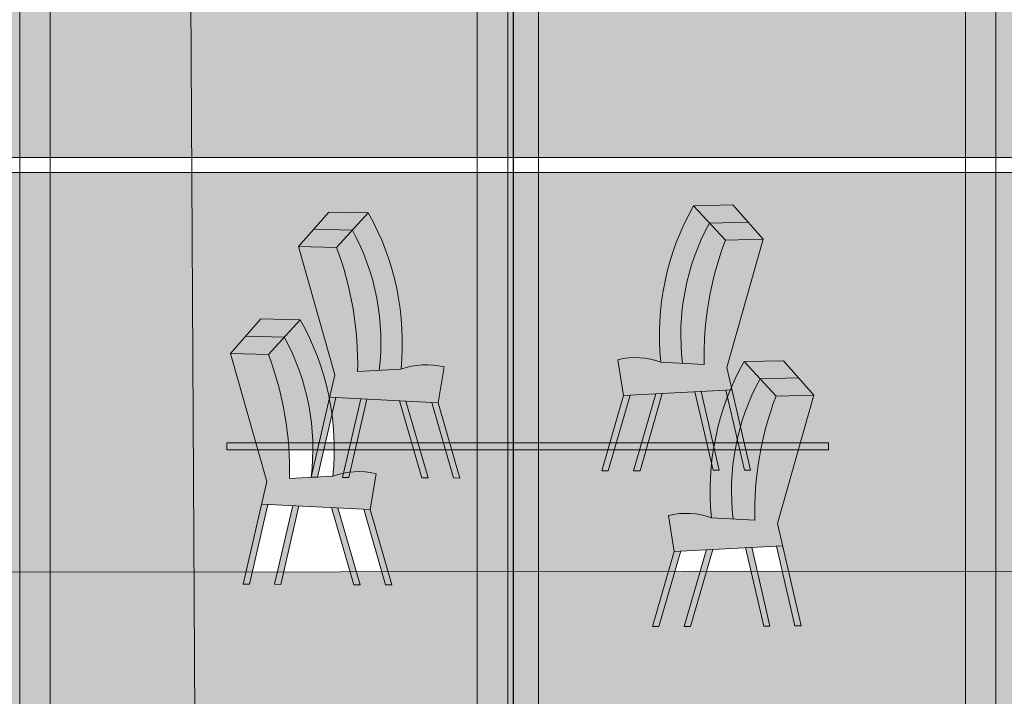
# Model space of a CAD drawing. Units: millimetres. Extents: x 11032 to 26788, y 3406 to 24505.
# Tile 14 of 78: x 17145 to 18758, y 7381 to 8490. Entities that reach past the tile are written whole.
import ezdxf

# ---------------------------------------------------------------- set-up
doc = ezdxf.new("R2010")
doc.units = ezdxf.units.MM
doc.header["$MEASUREMENT"] = 0
for name, color, linetype, lineweight in [('A-ANNO-DIMS', 2, 'Continuous', 18), ('A-FURN', 8, 'Continuous', 13), ('A-FURN-PATT', 8, 'Continuous', 13), ('A-GLAZ', 250, 'Continuous', 20), ('A-WALL-INTR', 8, 'Continuous', 18)]:
    doc.layers.add(name, color=color, linetype=linetype, lineweight=lineweight)
for name, color, linetype, lineweight, true_color in [('A-FNSH-INTR-PATT', 253, 'Continuous', 13, 0xc2b29b), ('A-GLAZ-FRAM-PATT', 250, 'Continuous', 13, 0x262627), ('A-WALL-INTR-PATT', 251, 'Continuous', 13, 0x6c6b6a)]:
    doc.layers.add(name, color=color, linetype=linetype, lineweight=lineweight, true_color=true_color)
doc.styles.get("Standard").update_dxf_attribs({"font": 'arial.ttf'})
doc.dimstyles.get("Standard").update_dxf_attribs({"dimtxt": 150, "dimasz": 100, "dimexe": 10, "dimexo": 5, "dimgap": 5, "dimtad": 0, "dimtih": 1, "dimtoh": 1, "dimdec": 0, "dimzin": 0, "dimdsep": 46, "dimtxsty": 'Standard', "dimcen": 0.09, "dimadec": 0, "dimazin": 0, "dimtfac": 1, "dimtdec": 0, "dimtofl": 0, "dimtmove": 0, "dimatfit": 3, "dimfxl": 1, "dimtolj": 1, "dimtzin": 0, "dimarcsym": 0})

# ---------------------------------------------------------------- blocks, each defined once
blk = doc.blocks.new('DINING-CHAIR-ELEV')
blk.add_line((228.7, 123.4), (51, 132.6))
for points in [[(0, 379.5), (49.4, 435.9), (114.1, 434.5)], [(61.2, 132.1), (30.8, 1.2), (20.5, 1.2), (59.5, 169.3), (0, 379.5), (61.9, 377.9)], [(111.9, 129.5), (82.1, 0.9), (71.8, 1), (101.8, 130)], [(165.3, 126.7), (201.8, 0.3), (212.2, 0.3), (175.8, 126.2)]]:
    blk.add_lwpolyline(points)
for points in [[(218.1, 124), (253.9, 0.1), (264.3, 0), (228.7, 123.4), (238.3, 182.2, 0.148451), (167.5, 178.3), (96.6, 174.5, 0.097012), (61.9, 377.9), (114.1, 434.5, -0.154833), (167.8, 178.5)], [(132, 176.4, 0.156877), (88, 406.2), (24.7, 407.7)]]:
    blk.add_lwpolyline(points, format="xyb")
blk = doc.blocks.new('DINING-TABLE-ELEV')
blk.add_lwpolyline([(0, 0), (986.1, 0), (986.1, 11.1), (0, 11.1)], close=True)
blk = doc.blocks.new('*D36')
at = {"layer": 'A-ANNO-DIMS', "color": 0, "lineweight": -2, "transparency": 16777216}
for p, q in [((12301.3, 17115.9), (12301.3, 24416.9)), ((25397.4, 4466.4), (25397.4, 24416.9)), ((12401.3, 24406.9), (18569.2, 24406.9)), ((25297.4, 24406.9), (19129.5, 24406.9))]:
    blk.add_line(p, q, dxfattribs=at)
at = {"layer": 'A-ANNO-DIMS', "color": 0, "transparency": 16777216}
for points in [[(12401.3, 24423.5), (12401.3, 24390.2), (12301.3, 24406.9)], [(25297.4, 24423.5), (25297.4, 24390.2), (25397.4, 24406.9)]]:
    blk.add_solid(points, dxfattribs=at)
at = {"layer": 'Defpoints', "color": 0, "transparency": 16777216}
for p in [(25397.4, 24406.9), (12301.3, 17110.9), (25397.4, 4461.4)]:
    blk.add_point(p, dxfattribs=at)
at = {"layer": 'A-ANNO-DIMS', "color": 0, "transparency": 16777216, "insert": (18849.3, 24406.9), "char_height": 150, "attachment_point": 5}
blk.add_mtext('\\A1;13096', dxfattribs=at)
blk = doc.blocks.new('*D37')
at = {"layer": 'A-ANNO-DIMS', "color": 0, "lineweight": -2, "transparency": 16777216}
for p, q in [((18087.7, 23450.4), (11334.8, 23450.4)), ((11344.8, 23350.4), (11344.8, 14037.5)), ((11344.8, 4561.4), (11344.8, 13874.3)), ((12927.7, 4461.4), (11334.8, 4461.4))]:
    blk.add_line(p, q, dxfattribs=at)
at = {"layer": 'A-ANNO-DIMS', "color": 0, "transparency": 16777216}
for points in [[(11328.1, 23350.4), (11361.4, 23350.4), (11344.8, 23450.4)], [(11328.1, 4561.4), (11361.4, 4561.4), (11344.8, 4461.4)]]:
    blk.add_solid(points, dxfattribs=at)
at = {"layer": 'Defpoints', "color": 0, "transparency": 16777216}
for p in [(11344.8, 23450.4), (18092.7, 23450.4), (12932.7, 4461.4)]:
    blk.add_point(p, dxfattribs=at)
at = {"layer": 'A-ANNO-DIMS', "color": 0, "transparency": 16777216, "insert": (11344.8, 13955.9), "char_height": 150, "attachment_point": 5}
blk.add_mtext('\\A1;18989', dxfattribs=at)
blk = doc.blocks.new('*D49')
at = {"layer": 'A-ANNO-DIMS', "color": 0, "lineweight": -2, "transparency": 16777216}
for p, q in [((17953.5, 10206.4), (17953.5, 3494.9)), ((14996.4, 6406.4), (14996.4, 3494.9)), ((15096.4, 3504.9), (16244.7, 3504.9)), ((17853.5, 3504.9), (16705.2, 3504.9))]:
    blk.add_line(p, q, dxfattribs=at)
at = {"layer": 'A-ANNO-DIMS', "color": 0, "transparency": 16777216}
for points in [[(15096.4, 3521.6), (15096.4, 3488.2), (14996.4, 3504.9)], [(17853.5, 3521.6), (17853.5, 3488.2), (17953.5, 3504.9)]]:
    blk.add_solid(points, dxfattribs=at)
at = {"layer": 'Defpoints', "color": 0, "transparency": 16777216}
for p in [(17953.5, 10211.4), (14996.4, 6411.4), (17953.5, 3504.9)]:
    blk.add_point(p, dxfattribs=at)
at = {"layer": 'A-ANNO-DIMS', "color": 0, "transparency": 16777216, "insert": (16474.9, 3504.9), "char_height": 150, "attachment_point": 5}
blk.add_mtext('\\A1;2957', dxfattribs=at)
blk = doc.blocks.new('*D50')
at = {"layer": 'A-ANNO-DIMS', "color": 0, "lineweight": -2, "transparency": 16777216}
for p, q in [((19697.4, 16000.7), (19697.4, 3494.9)), ((17953.5, 10206.4), (17953.5, 3494.9)), ((18053.5, 3504.9), (18603.8, 3504.9)), ((19597.4, 3504.9), (19047, 3504.9))]:
    blk.add_line(p, q, dxfattribs=at)
at = {"layer": 'A-ANNO-DIMS', "color": 0, "transparency": 16777216}
for points in [[(18053.5, 3521.6), (18053.5, 3488.2), (17953.5, 3504.9)], [(19597.4, 3521.6), (19597.4, 3488.2), (19697.4, 3504.9)]]:
    blk.add_solid(points, dxfattribs=at)
at = {"layer": 'Defpoints', "color": 0, "transparency": 16777216}
for p in [(19697.4, 16005.7), (17953.5, 10211.4), (19697.4, 3504.9)]:
    blk.add_point(p, dxfattribs=at)
at = {"layer": 'A-ANNO-DIMS', "color": 0, "transparency": 16777216, "insert": (18825.4, 3504.9), "char_height": 150, "attachment_point": 5}
blk.add_mtext('\\A1;1744', dxfattribs=at)
blk = doc.blocks.new('*D57')
at = {"layer": 'A-ANNO-DIMS', "color": 0, "lineweight": -2, "transparency": 16777216}
for p, q in [((14994.7, 7266.4), (14994.7, 24416.9)), ((20894.7, 7266.4), (20894.7, 24416.9)), ((15094.7, 24406.9), (17716, 24406.9)), ((20794.7, 24406.9), (18173.4, 24406.9))]:
    blk.add_line(p, q, dxfattribs=at)
at = {"layer": 'A-ANNO-DIMS', "color": 0, "transparency": 16777216}
for points in [[(15094.7, 24423.5), (15094.7, 24390.2), (14994.7, 24406.9)], [(20794.7, 24423.5), (20794.7, 24390.2), (20894.7, 24406.9)]]:
    blk.add_solid(points, dxfattribs=at)
at = {"layer": 'Defpoints', "color": 0, "transparency": 16777216}
for p in [(20894.7, 24406.9), (14994.7, 7261.4), (20894.7, 7261.4)]:
    blk.add_point(p, dxfattribs=at)
at = {"layer": 'A-ANNO-DIMS', "color": 0, "transparency": 16777216, "insert": (17944.7, 24406.9), "char_height": 150, "attachment_point": 5}
blk.add_mtext('\\A1;5900', dxfattribs=at)
blk = doc.blocks.new('*D66')
at = {"layer": 'A-ANNO-DIMS', "color": 0, "lineweight": -2, "transparency": 16777216}
for p, q in [((16725.9, 10296), (16725.9, 3494.9)), ((19150.9, 10296), (19150.9, 3494.9)), ((16825.9, 3504.9), (17707.6, 3504.9)), ((19050.9, 3504.9), (18169.3, 3504.9))]:
    blk.add_line(p, q, dxfattribs=at)
at = {"layer": 'A-ANNO-DIMS', "color": 0, "transparency": 16777216}
for points in [[(16825.9, 3521.6), (16825.9, 3488.2), (16725.9, 3504.9)], [(19050.9, 3521.6), (19050.9, 3488.2), (19150.9, 3504.9)]]:
    blk.add_solid(points, dxfattribs=at)
at = {"layer": 'Defpoints', "color": 0, "transparency": 16777216}
for p in [(16725.9, 10301), (19150.9, 10301), (19150.9, 3504.9)]:
    blk.add_point(p, dxfattribs=at)
at = {"layer": 'A-ANNO-DIMS', "color": 0, "transparency": 16777216, "insert": (17938.4, 3504.9), "char_height": 150, "attachment_point": 5}
blk.add_mtext('\\A1;2425', dxfattribs=at)
blk = doc.blocks.new('*D69')
at = {"layer": 'A-ANNO-DIMS', "color": 0, "lineweight": -2, "transparency": 16777216}
for p, q in [((13957, 9938), (14057, 9938)), ((14057, 9938), (15432.5, 8991)), ((17944.6, 7261.4), (17944.8, 7261.4)), ((17944.7, 7261.3), (17944.7, 7261.5))]:
    blk.add_line(p, q, dxfattribs=at)
at = {"layer": 'A-ANNO-DIMS', "color": 0, "transparency": 16777216}
blk.add_solid([(15442, 9004.7), (15423.1, 8977.2), (15514.9, 8934.2)], dxfattribs=at)
at = {"layer": 'Defpoints', "color": 0, "transparency": 16777216}
for p in [(15514.9, 8934.2), (17944.7, 7261.4)]:
    blk.add_point(p, dxfattribs=at)
at = {"layer": 'A-ANNO-DIMS', "color": 0, "transparency": 16777216, "insert": (13494, 9938), "char_height": 150, "attachment_point": 5}
blk.add_mtext('\\A1;2X R2950', dxfattribs=at)
blk = doc.blocks.new('*D70')
at = {"layer": 'A-ANNO-DIMS', "color": 0, "lineweight": -2, "transparency": 16777216}
for p, q in [((18044.7, 11901.4), (17944.7, 11901.4)), ((17944.7, 11901.4), (17944.7, 10261.4)), ((17944.6, 7261.4), (17944.8, 7261.4)), ((17944.7, 7261.3), (17944.7, 7261.5))]:
    blk.add_line(p, q, dxfattribs=at)
at = {"layer": 'A-ANNO-DIMS', "color": 0, "transparency": 16777216}
blk.add_solid([(17928, 10261.4), (17961.4, 10261.4), (17944.7, 10161.4)], dxfattribs=at)
at = {"layer": 'Defpoints', "color": 0, "transparency": 16777216}
for p in [(17944.7, 10161.4), (17944.7, 7261.4)]:
    blk.add_point(p, dxfattribs=at)
at = {"layer": 'A-ANNO-DIMS', "color": 0, "transparency": 16777216, "insert": (18345.2, 11901.4), "char_height": 150, "attachment_point": 5}
blk.add_mtext('\\A1;R2900', dxfattribs=at)

msp = doc.modelspace()

# ---------------------------------------------------------------- hatches: boundary and pattern name
at = {"layer": 'A-FNSH-INTR-PATT'}
h = msp.add_hatch(dxfattribs=at)
h.set_pattern_fill('AR-SAND', color=256, scale=30, angle=45, style=0)
h.paths.add_polyline_path([(17894.704, 10061.399), (17417.202, 10027.292), (17426.61, 8264.696), (17894.704, 8264.696)])
h.paths.add_polyline_path([(18694.704, 10011.399), (17994.704, 10061.399), (17994.704, 8264.696), (18694.704, 8264.696)])
h.paths.add_polyline_path([(19494.704, 9712.419, 0.04762013), (19003.004, 9961.399), (18794.704, 9961.399), (18794.704, 8264.696), (19494.704, 8264.696)])
at = {"layer": 'A-FURN-PATT'}
h = msp.add_hatch(color=256, dxfattribs=at)
h.set_gradient(color1=(82, 15, 16), color2=(153, 0, 38), name='CURVED')
h.paths.add_polyline_path([(16952.125, 8119), (16926.017, 8147.32, 0.15687748), (16881.989, 7917.509), (16917.415, 7915.583, -0.09701208)], flags=0)
h.paths.add_polyline_path([(16899.908, 8175.64), (16964.58, 8177.046), (17014.03, 8120.657), (16954.484, 7910.365), (16972.017, 7834.84), (16977.75, 7834.965), (17027.199, 7778.576), (16967.653, 7568.284), (17006.665, 7400.238), (16996.411, 7400.187), (16966.016, 7531.114), (16925.439, 7529.018), (16955.395, 7399.983), (16945.141, 7399.932), (16915.295, 7528.494), (16861.916, 7525.736), (16825.435, 7399.337), (16815.012, 7399.285), (16851.35, 7525.19), (16809.087, 7523.007), (16773.319, 7399.078), (16762.896, 7399.026), (16798.521, 7522.461), (16788.882, 7581.207, -0.14766935), (16859.382, 7577.482, -0.15281323), (16911.41, 7830.579), (16902.125, 7870.575), (16848.746, 7867.817), (16830.506, 7804.617), (16830.506, 7793.515), (16827.302, 7793.515), (16812.265, 7741.418), (16801.842, 7741.366), (16816.893, 7793.515), (16775.261, 7793.515), (16760.15, 7741.159), (16749.727, 7741.107), (16764.853, 7793.515), (16650.704, 7793.515), (16662.994, 7750.932), (16652.571, 7750.983), (16640.296, 7793.515), (16598.663, 7793.515), (16610.879, 7751.191), (16600.455, 7751.242), (16588.255, 7793.515), (16490.425, 7793.515), (16480.749, 7751.837), (16470.495, 7751.888), (16480.159, 7793.515), (16443.833, 7793.515, -0.10940509), (16465.746, 7607.731, -0.14766935), (16536.246, 7611.456), (16526.606, 7552.71), (16562.232, 7429.275), (16551.809, 7429.327), (16516.041, 7553.255), (16473.778, 7555.439), (16510.116, 7429.534), (16499.693, 7429.586), (16463.212, 7555.985), (16409.833, 7558.743), (16379.987, 7430.181), (16369.733, 7430.232), (16394.704, 7537.793), (16394.704, 7559.524), (16359.112, 7561.363), (16328.717, 7430.435), (16318.463, 7430.486), (16344.704, 7543.521), (16344.704, 7643.635), (16302.264, 7793.515), (16205.738, 7793.515), (16227.021, 7719.773), (16216.598, 7719.825), (16195.329, 7793.515), (16153.697, 7793.515), (16174.905, 7720.032), (16164.482, 7720.084), (16143.289, 7793.515), (15844.423, 7793.515), (15844.423, 7804.617), (16140.084, 7804.617), (16128.001, 7846.483), (16191.395, 7843.208), (16201.035, 7901.954, 0.14845082), (16130.184, 7898.102), (16059.333, 7894.25, 0.09701208), (16024.622, 8097.666), (16076.839, 8154.307, -0.15483335), (16130.535, 7898.229, -0.14766935), (16201.035, 7901.954), (16191.395, 7843.208), (16202.533, 7804.617), (16299.12, 7804.617), (16297.929, 7808.825), (16347.378, 7865.214), (16412.05, 7863.808, -0.02954963), (16434.494, 7817.915), (16458.237, 7920.19), (16398.691, 8130.481), (16448.141, 8186.871), (16512.813, 8185.465, -0.15483335), (16566.508, 7929.387, -0.14766935), (16637.008, 7933.112), (16627.369, 7874.366), (16647.499, 7804.617), (16742.939, 7804.617), (16741.107, 8264.696), (17994.704, 8264.696), (17994.704, 7796.661), (18112.02, 7796.661), (18134.447, 7874.366), (18124.807, 7933.112, -0.14766935), (18195.307, 7929.387, -0.15483335), (18249.003, 8185.465), (18313.675, 8186.871), (18363.124, 8130.481), (18303.578, 7920.19), (18311.087, 7887.847, -0.02730168), (18332.016, 7930.161), (18396.688, 7931.567), (18446.137, 7875.177), (18423.905, 7796.661), (18470.25, 7796.661), (18470.25, 7785.559), (18420.761, 7785.559), (18386.591, 7664.886), (18425.604, 7496.839), (18415.35, 7496.788), (18384.955, 7627.716), (18344.377, 7625.62), (18374.333, 7496.584), (18364.079, 7496.533), (18334.233, 7625.095), (18280.854, 7622.338), (18244.373, 7495.938), (18233.95, 7495.887), (18270.288, 7621.792), (18228.026, 7619.608), (18192.257, 7495.679), (18181.834, 7495.628), (18217.46, 7619.062), (18207.82, 7677.808, -0.14766935), (18278.32, 7674.083, -0.05141811), (18278.516, 7762.821), (18273.237, 7785.559), (18171.265, 7785.559), (18161.36, 7751.242), (18150.937, 7751.191), (18160.856, 7785.559), (18119.224, 7785.559), (18109.244, 7750.983), (18098.821, 7750.932), (18108.815, 7785.559), (17852.794, 7785.559), (17866.18, 7739.181), (17855.756, 7739.233), (17842.386, 7785.559), (17800.753, 7785.559), (17814.064, 7739.44), (17803.641, 7739.492), (17790.345, 7785.559), (17694.491, 7785.559), (17685.986, 7748.922, -0.08827454), (17728.687, 7746.171), (17719.047, 7687.425), (17754.673, 7563.99), (17744.25, 7564.042), (17708.482, 7687.971), (17666.219, 7690.154), (17702.557, 7564.249), (17692.134, 7564.301), (17655.653, 7690.7), (17602.274, 7693.458), (17572.428, 7564.896), (17562.174, 7564.947), (17592.13, 7693.982), (17551.553, 7696.078), (17521.158, 7565.151), (17510.903, 7565.202), (17549.916, 7733.248), (17535.103, 7785.559), (17484.167, 7785.559), (17484.167, 7796.661), (17531.96, 7796.661), (17490.37, 7943.54), (17539.819, 7999.929), (17604.491, 7998.523, -0.08024859), (17652.289, 7869.096), (17661.422, 7908.439), (17601.876, 8118.731), (17651.326, 8175.12), (17715.998, 8173.714, -0.15483335), (17769.694, 7917.637, -0.14766935), (17840.194, 7921.361), (17830.554, 7862.615), (17849.59, 7796.661), (17894.704, 7796.661), (17894.704, 8239.696), (16741.207, 8239.696), (16742.939, 7804.617), (16768.057, 7804.617), (16785.352, 7864.542), (16775.713, 7923.288, -0.14766935), (16846.212, 7919.563, -0.15483335)], flags=17)
h.paths.add_polyline_path([(16899.908, 8175.64), (16964.58, 8177.046), (17014.03, 8120.657), (16954.484, 7910.365), (16993.496, 7742.318), (16983.242, 7742.267), (16952.847, 7873.195), (16912.27, 7871.099), (16942.225, 7742.064), (16931.971, 7742.013), (16902.125, 7870.575), (16848.746, 7867.817), (16812.265, 7741.418), (16801.842, 7741.366), (16838.181, 7867.271), (16795.918, 7865.087), (16760.15, 7741.159), (16749.727, 7741.107), (16785.352, 7864.542), (16775.713, 7923.288, -0.14766935), (16846.212, 7919.563, -0.15483335)], flags=0)
h.paths.add_polyline_path([(16899.908, 8175.64), (16964.58, 8177.046), (17014.03, 8120.657), (16954.484, 7910.365), (16972.017, 7834.84), (16977.75, 7834.965), (17027.199, 7778.576), (16967.653, 7568.284), (17006.665, 7400.238), (16996.411, 7400.187), (16966.016, 7531.114), (16925.439, 7529.018), (16955.395, 7399.983), (16945.141, 7399.932), (16915.295, 7528.494), (16861.916, 7525.736), (16825.435, 7399.337), (16815.012, 7399.285), (16851.35, 7525.19), (16809.087, 7523.007), (16773.319, 7399.078), (16762.896, 7399.026), (16798.521, 7522.461), (16788.882, 7581.207, -0.14766935), (16859.382, 7577.482, -0.15281323), (16911.41, 7830.579), (16902.125, 7870.575), (16848.746, 7867.817), (16830.506, 7804.617), (16830.506, 7793.515), (16827.302, 7793.515), (16812.265, 7741.418), (16801.842, 7741.366), (16816.893, 7793.515), (16775.261, 7793.515), (16760.15, 7741.159), (16749.727, 7741.107), (16764.853, 7793.515), (16650.704, 7793.515), (16662.994, 7750.932), (16652.571, 7750.983), (16640.296, 7793.515), (16598.663, 7793.515), (16610.879, 7751.191), (16600.455, 7751.242), (16588.255, 7793.515), (16490.425, 7793.515), (16480.749, 7751.837), (16470.495, 7751.888), (16480.159, 7793.515), (16443.833, 7793.515, -0.10940509), (16465.746, 7607.731, -0.14766935), (16536.246, 7611.456), (16526.606, 7552.71), (16562.232, 7429.275), (16551.809, 7429.327), (16516.041, 7553.255), (16473.778, 7555.439), (16510.116, 7429.534), (16499.693, 7429.586), (16463.212, 7555.985), (16409.833, 7558.743), (16379.987, 7430.181), (16369.733, 7430.232), (16394.704, 7537.793), (16394.704, 7559.524), (16359.112, 7561.363), (16328.717, 7430.435), (16318.463, 7430.486), (16344.704, 7543.521), (16344.704, 7643.635), (16302.264, 7793.515), (16205.738, 7793.515), (16227.021, 7719.773), (16216.598, 7719.825), (16195.329, 7793.515), (16153.697, 7793.515), (16174.905, 7720.032), (16164.482, 7720.084), (16143.289, 7793.515), (15844.423, 7793.515), (15844.423, 7804.617), (16140.084, 7804.617), (16128.001, 7846.483), (16191.395, 7843.208), (16201.035, 7901.954, 0.14845082), (16130.184, 7898.102), (16059.333, 7894.25, 0.09701208), (16024.622, 8097.666), (16076.839, 8154.307, -0.15483335), (16130.535, 7898.229, -0.14766935), (16201.035, 7901.954), (16191.395, 7843.208), (16202.533, 7804.617), (16299.12, 7804.617), (16297.929, 7808.825), (16347.378, 7865.214), (16412.05, 7863.808, -0.02954963), (16434.494, 7817.915), (16458.237, 7920.19), (16398.691, 8130.481), (16448.141, 8186.871), (16512.813, 8185.465, -0.15483335), (16566.508, 7929.387, -0.14766935), (16637.008, 7933.112), (16627.369, 7874.366), (16647.499, 7804.617), (16742.939, 7804.617), (16741.207, 8239.696), (16741.107, 8264.696), (17994.704, 8264.696), (17994.704, 7796.661), (18112.02, 7796.661), (18134.447, 7874.366), (18124.807, 7933.112, -0.14766935), (18195.307, 7929.387, -0.15483335), (18249.003, 8185.465), (18313.675, 8186.871), (18363.124, 8130.481), (18303.578, 7920.19), (18311.087, 7887.847, -0.02730168), (18332.016, 7930.161), (18396.688, 7931.567), (18446.137, 7875.177), (18423.905, 7796.661), (18470.25, 7796.661), (18470.25, 7785.559), (18420.761, 7785.559), (18386.591, 7664.886), (18425.604, 7496.839), (18415.35, 7496.788), (18384.955, 7627.716), (18344.377, 7625.62), (18374.333, 7496.584), (18364.079, 7496.533), (18334.233, 7625.095), (18280.854, 7622.338), (18244.373, 7495.938), (18233.95, 7495.887), (18270.288, 7621.792), (18228.026, 7619.608), (18192.257, 7495.679), (18181.834, 7495.628), (18217.46, 7619.062), (18207.82, 7677.808, -0.14766935), (18278.32, 7674.083, -0.05141811), (18278.516, 7762.821), (18273.237, 7785.559), (18171.265, 7785.559), (18161.36, 7751.242), (18150.937, 7751.191), (18160.856, 7785.559), (18119.224, 7785.559), (18109.244, 7750.983), (18098.821, 7750.932), (18108.815, 7785.559), (17852.794, 7785.559), (17866.18, 7739.181), (17855.756, 7739.233), (17842.386, 7785.559), (17800.753, 7785.559), (17814.064, 7739.44), (17803.641, 7739.492), (17790.345, 7785.559), (17694.491, 7785.559), (17685.986, 7748.922, -0.08827454), (17728.687, 7746.171), (17719.047, 7687.425), (17754.673, 7563.99), (17744.25, 7564.042), (17708.482, 7687.971), (17666.219, 7690.154), (17702.557, 7564.249), (17692.134, 7564.301), (17655.653, 7690.7), (17602.274, 7693.458), (17572.428, 7564.896), (17562.174, 7564.947), (17592.13, 7693.982), (17551.553, 7696.078), (17521.158, 7565.151), (17510.903, 7565.202), (17549.916, 7733.248), (17535.103, 7785.559), (17484.167, 7785.559), (17484.167, 7796.661), (17531.96, 7796.661), (17490.37, 7943.54), (17539.819, 7999.929), (17604.491, 7998.523, -0.08024859), (17652.289, 7869.096), (17661.422, 7908.439), (17601.876, 8118.731), (17651.326, 8175.12), (17715.998, 8173.714, -0.15483335), (17769.694, 7917.637, -0.14766935), (17840.194, 7921.361), (17830.554, 7862.615), (17849.59, 7796.661), (17894.704, 7796.661), (17894.704, 8239.696), (16741.207, 8239.696), (16742.939, 7804.617), (16768.057, 7804.617), (16785.352, 7864.542), (16775.713, 7923.288, -0.14766935), (16846.212, 7919.563, -0.15483335)], flags=17)
h = msp.add_hatch(color=256, dxfattribs=at)
h.set_gradient(color1=(82, 15, 16), color2=(153, 0, 38), name='CURVED')
h.paths.add_polyline_path([(17578.383, 7970.203), (17552.274, 7941.883, -0.06969308), (17585.247, 7796.661), (17625.121, 7796.661, 0.11927475)], flags=16)
h.paths.add_polyline_path([(17552.274, 7941.883), (17490.37, 7943.54), (17531.96, 7796.661), (17585.247, 7796.661, 0.06969308)], flags=16)
h.paths.add_polyline_path([(17604.491, 7998.523), (17539.819, 7999.929), (17515.094, 7971.734), (17578.383, 7970.203)], flags=17)
h.paths.add_polyline_path([(17578.383, 7970.203), (17515.094, 7971.734), (17490.37, 7943.54), (17552.274, 7941.883)], flags=16)
h.paths.add_polyline_path([(17604.491, 7998.523), (17578.383, 7970.203, -0.11927475), (17625.121, 7796.661), (17635.473, 7796.661), (17652.289, 7869.096, 0.08024859)], flags=17)
h.paths.add_polyline_path([(17586.067, 7785.559), (17535.103, 7785.559), (17549.916, 7733.248), (17541.408, 7696.602), (17719.047, 7687.425), (17728.687, 7746.171, 0.08827454), (17685.986, 7748.922), (17683.935, 7740.087), (17673.681, 7740.138), (17675.331, 7747.247, 0.03725953), (17657.836, 7742.318), (17632.807, 7740.958), (17632.664, 7740.341), (17622.41, 7740.392), (17586.985, 7738.466, 0.02194752)], flags=16)
h.paths.add_polyline_path([(17625.245, 7785.559), (17586.067, 7785.559, -0.02194752), (17586.985, 7738.466), (17622.41, 7740.392, 0.02963862)], flags=16)
h.paths.add_polyline_path([(17660.371, 7785.559), (17643.162, 7785.559), (17632.807, 7740.958), (17658.176, 7742.337, 0.02502642)], flags=16)
h.paths.add_polyline_path([(17656.551, 7843.232), (17645.739, 7796.661), (17660.237, 7796.661, 0.02701767)], flags=16)
h.paths.add_polyline_path([(17840.194, 7921.361, 0.14845082), (17769.342, 7917.509), (17698.491, 7913.657, 0.09701208), (17663.781, 8117.074), (17601.876, 8118.731), (17661.422, 7908.439), (17652.915, 7871.793), (17830.554, 7862.615)], flags=17)
h.paths.add_polyline_path([(17689.889, 8145.394), (17663.781, 8117.074, -0.09701208), (17698.491, 7913.657), (17733.917, 7915.583, 0.15687748)], flags=17)
h.paths.add_polyline_path([(17840.194, 7921.361), (17830.554, 7862.615), (17849.59, 7796.661), (18112.02, 7796.661), (18134.447, 7874.366), (18124.807, 7933.112, -0.14766935), (18195.307, 7929.387, -0.15483335), (18249.003, 8185.465), (18301.22, 8128.825), (18363.124, 8130.481), (18303.578, 7920.19), (18311.087, 7887.847, -0.02730168), (18332.016, 7930.161), (18396.688, 7931.567), (18446.137, 7875.177), (18423.905, 7796.661), (18470.25, 7796.661), (18470.25, 7785.559), (18420.761, 7785.559), (18386.591, 7664.886), (18425.604, 7496.839), (18415.35, 7496.788), (18384.955, 7627.716), (18344.377, 7625.62), (18374.333, 7496.584), (18364.079, 7496.533), (18334.233, 7625.095), (18280.854, 7622.338), (18244.373, 7495.938), (18233.95, 7495.887), (18270.288, 7621.792), (18228.026, 7619.608), (18192.257, 7495.679), (18181.834, 7495.628), (18217.46, 7619.062), (18207.82, 7677.808, -0.14766935), (18278.32, 7674.083, -0.05141811), (18278.516, 7762.821), (18273.237, 7785.559), (18171.265, 7785.559), (18161.36, 7751.242), (18150.937, 7751.191), (18160.856, 7785.559), (18119.224, 7785.559), (18109.244, 7750.983), (18098.821, 7750.932), (18108.815, 7785.559), (17852.794, 7785.559), (17866.18, 7739.181), (17855.756, 7739.233), (17842.386, 7785.559), (17800.753, 7785.559), (17814.064, 7739.44), (17803.641, 7739.492), (17790.345, 7785.559), (17694.491, 7785.559), (17685.986, 7748.922, -0.08827454), (17728.687, 7746.171), (17719.047, 7687.425), (17754.673, 7563.99), (17744.25, 7564.042), (17708.482, 7687.971), (17666.219, 7690.154), (17702.557, 7564.249), (17692.134, 7564.301), (17655.653, 7690.7), (17602.274, 7693.458), (17572.428, 7564.896), (17562.174, 7564.947), (17592.13, 7693.982), (17551.553, 7696.078), (17521.158, 7565.151), (17510.903, 7565.202), (17549.916, 7733.248), (17535.103, 7785.559), (17484.167, 7785.559), (17484.167, 7796.661), (17531.96, 7796.661), (17490.37, 7943.54), (17515.094, 7971.734), (17539.819, 7999.929), (17604.491, 7998.523, -0.08024859), (17652.289, 7869.096), (17661.422, 7908.439), (17601.876, 8118.731), (17663.781, 8117.074), (17715.998, 8173.714, -0.15483335), (17769.694, 7917.637, -0.14766935)])
h = msp.add_hatch(color=256, dxfattribs=at)
h.set_gradient(color1=(82, 15, 16), color2=(153, 0, 38), name='CURVED')
h.paths.add_polyline_path([(17689.889, 8145.394), (17626.601, 8146.925), (17601.876, 8118.731), (17663.781, 8117.074)])
h.paths.add_polyline_path([(17715.998, 8173.714), (17651.326, 8175.12), (17626.601, 8146.925), (17689.889, 8145.394)])
h.paths.add_polyline_path([(18313.675, 8186.871), (18249.003, 8185.465), (18275.111, 8157.145), (18338.4, 8158.676)])
h.paths.add_polyline_path([(18338.4, 8158.676), (18275.111, 8157.145), (18301.22, 8128.825), (18363.124, 8130.481)])
h = msp.add_hatch(color=256, dxfattribs=at)
h.set_gradient(color1=(82, 15, 16), color2=(153, 0, 38), name='CURVED')
h.paths.add_polyline_path([(17663.781, 8117.074), (17601.876, 8118.731), (17661.422, 7908.439), (17652.915, 7871.793), (17830.554, 7862.615), (17840.194, 7921.361, 0.14845082), (17769.342, 7917.509), (17698.491, 7913.657, 0.09701208)])
h.paths.add_polyline_path([(17689.889, 8145.394), (17663.781, 8117.074, -0.09701208), (17698.491, 7913.657), (17733.917, 7915.583, 0.15687748)])
h.paths.add_polyline_path([(17578.383, 7970.203), (17515.094, 7971.734), (17490.37, 7943.54), (17552.274, 7941.883)])
h.paths.add_polyline_path([(17604.491, 7998.523), (17539.819, 7999.929), (17515.094, 7971.734), (17578.383, 7970.203)])
h.paths.add_polyline_path([(17604.491, 7998.523), (17578.383, 7970.203, -0.11927475), (17625.121, 7796.661), (17635.473, 7796.661), (17652.289, 7869.096, 0.08024859)])
h.paths.add_polyline_path([(17578.383, 7970.203), (17552.274, 7941.883, -0.06969308), (17585.247, 7796.661), (17625.121, 7796.661, 0.11927475)])
h.paths.add_polyline_path([(17552.274, 7941.883), (17490.37, 7943.54), (17531.96, 7796.661), (17585.247, 7796.661, 0.06969308)])
h.paths.add_polyline_path([(17728.687, 7746.171, 0.08827454), (17685.986, 7748.922), (17683.935, 7740.087), (17673.681, 7740.138), (17675.331, 7747.247, 0.03725953), (17657.836, 7742.318), (17632.807, 7740.958), (17632.664, 7740.341), (17622.41, 7740.392), (17586.985, 7738.466, 0.02194752), (17586.067, 7785.559), (17535.103, 7785.559), (17549.916, 7733.248), (17541.408, 7696.602), (17719.047, 7687.425)])
at = {"layer": 'A-GLAZ-FRAM-PATT'}
h = msp.add_hatch(color=256, dxfattribs=at)
h.paths.add_polyline_path([(17944.704, 7311.399), (16344.704, 7311.399), (16344.704, 7261.399), (17944.704, 7261.399)], flags=17)
h.paths.add_polyline_path([(16344.704, 7311.399), (15045.135, 7311.399, -0.98290472), (20844.273, 7311.399), (19544.704, 7311.399), (19544.704, 7261.399), (20894.704, 7261.399, 0.51484406), (16985.951, 10051.255, 0.32026791), (14994.704, 7261.399), (16344.704, 7261.399)])
h.paths.add_polyline_path([(18744.704, 7311.399), (17944.704, 7311.399), (17944.704, 7261.399), (18744.704, 7261.399)], flags=17)
h.paths.add_polyline_path([(19544.704, 7311.399), (18744.704, 7311.399), (18744.704, 7261.399), (19544.704, 7261.399)], flags=17)
h.paths.add_polyline_path([(18694.704, 7361.399), (17994.704, 7361.399), (17994.704, 7311.399), (18694.704, 7311.399)], flags=17)
h.paths.add_polyline_path([(18744.704, 7361.399), (18694.704, 7361.399), (18694.704, 7311.399), (18744.704, 7311.399)], flags=17)
h.paths.add_polyline_path([(17194.704, 7361.399), (17144.704, 7361.399), (17144.704, 7311.399), (17194.704, 7311.399)], flags=17)
h.paths.add_polyline_path([(17431.432, 7361.399), (17194.704, 7361.399), (17194.704, 7311.399), (17431.699, 7311.399)], flags=17)
h.paths.add_polyline_path([(17894.704, 7361.399), (17431.432, 7361.399), (17431.699, 7311.399), (17894.704, 7311.399)], flags=17)
h.paths.add_polyline_path([(17944.704, 7361.399), (17894.704, 7361.399), (17894.704, 7311.399), (17944.704, 7311.399)], flags=17)
h.paths.add_polyline_path([(17994.704, 7361.399), (17944.704, 7361.399), (17944.704, 7311.399), (17994.704, 7311.399)], flags=17)
h = msp.add_hatch(color=256, dxfattribs=at)
h.paths.add_polyline_path([(17944.704, 10161.399, 0.06998554), (17144.704, 10048.871), (17144.704, 8264.696), (17194.704, 8264.696), (17194.704, 10011.399), (17894.704, 10061.399), (17894.704, 8264.696), (17944.704, 8264.696)])
h.paths.add_polyline_path([(17950.351, 10161.394), (17944.704, 8842.998), (17944.704, 8264.696), (17994.704, 8264.696), (17994.704, 10061.399), (18694.704, 10011.399), (18694.704, 8264.696), (18744.704, 8264.696), (18744.704, 10048.871, 0.06949637)])
h = msp.add_hatch(color=256, dxfattribs=at)
h.paths.add_polyline_path([(16394.704, 9712.419, 0.00513365), (16344.704, 9680.076), (16344.704, 7862.164), (16347.378, 7865.214), (16394.704, 7864.185)])
h.paths.add_polyline_path([(17144.704, 10048.871, 0.02352245), (16886.403, 9961.399), (17094.704, 9961.399), (17094.704, 8264.696), (17144.704, 8264.696)])
h.paths.add_polyline_path([(18794.704, 9961.399), (19003.004, 9961.399, 0.02352245), (18744.704, 10048.871), (18744.704, 8264.696), (18794.704, 8264.696)])
h.paths.add_polyline_path([(19544.704, 9680.076, 0.00513365), (19494.704, 9712.419), (19494.704, 7793.43), (19544.704, 7793.43)])
h = msp.add_hatch(color=256, dxfattribs=at)
h.paths.add_polyline_path([(16734.609, 9896.863, 0.03337538), (16394.704, 9712.419), (16394.704, 7804.617), (16431.407, 7804.617), (16458.237, 7920.19), (16398.691, 8130.481), (16448.141, 8186.871), (16512.813, 8185.465, -0.15483335), (16566.508, 7929.387, -0.14766935), (16637.008, 7933.112), (16627.369, 7874.366), (16647.499, 7804.617), (16742.939, 7804.617)])
h.paths.add_polyline_path([(17094.704, 9961.399), (16886.403, 9961.399, 0.01422214), (16734.609, 9896.863), (16741.107, 8264.696), (17094.704, 8264.696)])
h.paths.add_polyline_path([(17417.202, 10027.292), (17194.704, 10011.399), (17194.704, 8264.696), (17426.61, 8264.696)])
h.paths.add_polyline_path([(17144.704, 8239.696), (17094.704, 8239.696), (17094.704, 7361.399), (16394.704, 7361.399), (16394.704, 7493.572), (16379.987, 7430.181), (16369.733, 7430.232), (16394.704, 7537.793), (16394.704, 7559.524), (16359.112, 7561.363), (16344.704, 7499.3), (16344.704, 7311.399), (17144.704, 7311.399)])
h.paths.add_polyline_path([(17194.704, 8239.696), (17144.704, 8239.696), (17144.704, 7361.399), (17194.704, 7361.399)])
h = msp.add_hatch(color=256, dxfattribs=at)
h.paths.add_polyline_path([(17426.744, 8239.696), (17194.704, 8239.696), (17194.704, 7584.945), (17430.237, 7585.191)])
h.paths.add_polyline_path([(18694.704, 8239.696), (17994.704, 8239.696), (17994.704, 7796.661), (18112.02, 7796.661), (18134.447, 7874.366), (18124.807, 7933.112, -0.14766935), (18195.307, 7929.387, -0.15483335), (18249.003, 8185.465), (18313.675, 8186.871), (18363.124, 8130.481), (18303.578, 7920.19), (18311.087, 7887.847, -0.02730168), (18332.016, 7930.161), (18396.688, 7931.567), (18446.137, 7875.177), (18423.905, 7796.661), (18470.25, 7796.661), (18470.25, 7785.559), (18420.761, 7785.559), (18386.591, 7664.886), (18404.857, 7586.207), (18694.704, 7586.509)])
h.paths.add_polyline_path([(17894.704, 8239.696), (17426.744, 8239.696), (17430.237, 7585.191), (17515.565, 7585.28), (17549.916, 7733.248), (17535.103, 7785.559), (17484.167, 7785.559), (17484.167, 7796.661), (17531.96, 7796.661), (17490.37, 7943.54), (17539.819, 7999.929), (17604.491, 7998.523, -0.07861293), (17651.739, 7871.854), (17652.915, 7871.793), (17661.422, 7908.439), (17601.876, 8118.731), (17651.326, 8175.12), (17715.998, 8173.714, -0.15483335), (17769.694, 7917.637, -0.14766935), (17840.194, 7921.361), (17830.554, 7862.615), (17849.59, 7796.661), (17894.704, 7796.661)])
h.paths.add_polyline_path([(17894.704, 7785.559), (17852.794, 7785.559), (17866.18, 7739.181), (17855.756, 7739.233), (17842.386, 7785.559), (17800.753, 7785.559), (17814.064, 7739.44), (17803.641, 7739.492), (17790.345, 7785.559), (17694.491, 7785.559), (17685.986, 7748.922, -0.08827454), (17728.687, 7746.171), (17719.047, 7687.425), (17748.458, 7585.522), (17894.704, 7585.675)], flags=17)
h.paths.add_polyline_path([(18278.516, 7762.821), (18273.237, 7785.559), (18171.265, 7785.559), (18161.36, 7751.242), (18150.937, 7751.191), (18160.856, 7785.559), (18119.224, 7785.559), (18109.244, 7750.983), (18098.821, 7750.932), (18108.815, 7785.559), (17994.704, 7785.559), (17994.704, 7585.779), (18207.918, 7586.001), (18217.46, 7619.062), (18207.82, 7677.808, -0.14766935), (18278.32, 7674.083, -0.05141811)])
h = msp.add_hatch(color=256, dxfattribs=at)
h.paths.add_polyline_path([(17944.704, 8239.696), (17894.704, 8239.696), (17894.704, 7796.661), (17944.704, 7796.661)])
h.paths.add_polyline_path([(17994.704, 8239.696), (17944.704, 8239.696), (17944.704, 7796.661), (17994.704, 7796.661)])
h.paths.add_polyline_path([(17944.704, 7785.559), (17894.704, 7785.559), (17894.704, 7361.399), (17944.704, 7361.399)])
h.paths.add_polyline_path([(17994.704, 7785.559), (17944.704, 7785.559), (17944.704, 7361.399), (17994.704, 7361.399)])
h.paths.add_polyline_path([(18744.704, 8239.696), (18694.704, 8239.696), (18694.704, 7361.399), (18744.704, 7361.399)])
h.paths.add_polyline_path([(18794.704, 8239.696), (18744.704, 8239.696), (18744.704, 7311.399), (19544.704, 7311.399), (19544.704, 7613.382), (19531.043, 7566.052), (19520.62, 7566), (19544.704, 7649.444), (19544.704, 7691.272), (19514.696, 7689.722), (19494.704, 7620.453), (19494.704, 7361.399), (18794.704, 7361.399)])
at = {"layer": 'A-WALL-INTR-PATT'}
h = msp.add_hatch(color=256, dxfattribs=at)
h.paths.add_polyline_path([(19494.704, 9712.419, 0.04762013), (19003.004, 9961.399), (18794.704, 9961.399), (18794.704, 8264.696), (19494.704, 8264.696)])
h.paths.add_polyline_path([(18694.704, 10011.399), (17994.704, 10061.399), (17994.704, 8264.696), (18694.704, 8264.696)])
h.paths.add_polyline_path([(17894.704, 10061.399), (17417.202, 10027.292), (17426.61, 8264.696), (17894.704, 8264.696)])
h = msp.add_hatch(color=256, dxfattribs=at)
h.set_gradient(color1=(254, 234, 185), color2=(254, 204, 102), name='CURVED')
h.paths.add_polyline_path([(15260.167, 7582.928), (15062.56, 7582.722, 0.02345098), (15045.135, 7311.399), (15314.374, 7311.399)])
h.paths.add_polyline_path([(15413.095, 7583.087), (15260.167, 7582.928), (15314.374, 7311.399), (15467.334, 7311.399)])
h.paths.add_polyline_path([(15531.986, 7554.365), (15523.82, 7583.203), (15413.095, 7583.087), (15467.334, 7311.399), (15790.119, 7311.399), (15790.667, 7566.433), (15785.748, 7583.476), (15718.988, 7583.406), (15701.389, 7507.6), (15736.743, 7385.107), (15726.32, 7385.159), (15696.749, 7487.614), (15695.471, 7482.107), (15685.217, 7482.158), (15691.06, 7507.327), (15690.552, 7509.088), (15650.881, 7511.137), (15649.743, 7506.234), (15684.627, 7385.366), (15674.204, 7385.418), (15646.227, 7482.352), (15633.946, 7482.413), (15639.413, 7505.961), (15637.723, 7511.817), (15584.344, 7514.575), (15554.498, 7386.013), (15544.244, 7386.064), (15574.2, 7515.099), (15533.623, 7517.195), (15503.228, 7386.268), (15492.974, 7386.319)])
h.paths.add_polyline_path([(16344.704, 7499.3), (16328.717, 7430.435), (16318.463, 7430.486), (16344.704, 7543.521), (16344.704, 7584.059), (16080.595, 7583.783), (16085.615, 7566.39), (16075.192, 7566.442), (16070.19, 7583.773), (16028.57, 7583.729), (16033.5, 7566.649), (16023.077, 7566.701), (16018.165, 7583.718), (15907.156, 7583.603), (15903.371, 7567.296), (15893.116, 7567.347), (15896.888, 7583.592), (15855.814, 7583.549), (15852.409, 7568.882), (15877.716, 7481.201), (15867.293, 7481.253), (15844.553, 7560.041), (15844.691, 7311.399), (16344.704, 7311.399)])
h.paths.add_polyline_path([(15844.553, 7560.041), (15842.372, 7567.599), (15841.846, 7567.602), (15842.08, 7568.609), (15837.773, 7583.53), (15796.153, 7583.487), (15825.6, 7481.46), (15815.177, 7481.512), (15790.667, 7566.433), (15790.119, 7311.399), (15844.691, 7311.399)])
h.paths.add_polyline_path([(16394.704, 7493.572), (16379.987, 7430.181), (16369.733, 7430.232), (16394.704, 7537.793), (16394.704, 7559.524), (16359.112, 7561.363), (16344.704, 7499.3), (16344.704, 7311.399), (17144.704, 7311.399), (17144.704, 7584.893), (17094.704, 7584.841), (17094.704, 7361.399), (16394.704, 7361.399)])
h.paths.add_polyline_path([(17430.237, 7585.191), (17194.704, 7584.945), (17194.704, 7361.399), (17431.432, 7361.399)])
h.paths.add_polyline_path([(17894.704, 7585.675), (17748.458, 7585.522), (17754.673, 7563.99), (17744.25, 7564.042), (17738.053, 7585.511), (17696.433, 7585.468), (17702.557, 7564.249), (17692.134, 7564.301), (17686.028, 7585.457), (17577.175, 7585.344), (17572.428, 7564.896), (17562.174, 7564.947), (17566.907, 7585.333), (17525.833, 7585.29), (17521.158, 7565.151), (17510.903, 7565.202), (17515.565, 7585.28), (17430.237, 7585.191), (17431.432, 7361.399), (17894.704, 7361.399)])
h.paths.add_polyline_path([(18694.704, 7586.509), (18404.857, 7586.207), (18425.604, 7496.839), (18415.35, 7496.788), (18394.593, 7586.196), (18353.54, 7586.153), (18374.333, 7496.584), (18364.079, 7496.533), (18343.276, 7586.142), (18270.386, 7586.066), (18244.373, 7495.938), (18233.95, 7495.887), (18259.974, 7586.056), (18218.329, 7586.012), (18192.257, 7495.679), (18181.834, 7495.628), (18207.918, 7586.001), (17994.704, 7585.779), (17994.704, 7361.399), (18694.704, 7361.399)])
h.paths.add_polyline_path([(19317.979, 7532.562), (19264.6, 7535.319), (19234.754, 7406.757), (19224.5, 7406.808), (19254.456, 7535.844), (19213.879, 7537.94), (19183.484, 7407.012), (19173.23, 7407.063), (19212.242, 7575.11), (19208.862, 7587.045), (19127.433, 7586.96), (19124.467, 7576.487), (19163.48, 7408.44), (19153.225, 7408.389), (19122.83, 7539.317), (19082.253, 7537.22), (19112.209, 7408.185), (19101.955, 7408.134), (19072.109, 7536.696), (19035.898, 7534.825), (19044.517, 7497.701), (19034.262, 7497.65), (19025.754, 7534.301), (19018.73, 7533.938), (18982.249, 7407.539), (18971.826, 7407.487), (19008.164, 7533.392), (18985.177, 7532.205), (18993.246, 7497.447), (18982.992, 7497.396), (18975.033, 7531.681), (18965.902, 7531.209), (18930.133, 7407.28), (18919.71, 7407.228), (18955.336, 7530.663), (18946.129, 7586.771), (18889.236, 7586.712), (18863.286, 7496.801), (18852.863, 7496.749), (18878.825, 7586.701), (18837.179, 7586.657), (18811.17, 7496.542), (18800.747, 7496.49), (18826.768, 7586.647), (18794.704, 7586.613), (18794.704, 7361.399), (19494.704, 7361.399), (19494.704, 7587.343), (19485.145, 7587.333), (19478.928, 7565.793), (19468.505, 7565.741), (19473, 7581.318), (19466.812, 7581.349), (19465.091, 7587.312), (19423.471, 7587.269), (19425.12, 7581.556), (19414.696, 7581.608), (19413.066, 7587.258), (19390.882, 7587.235), (19381.373, 7529.286), (19416.999, 7405.852), (19406.576, 7405.903), (19370.808, 7529.832), (19328.545, 7532.016), (19364.883, 7406.111), (19354.46, 7406.162)])
h.paths.add_polyline_path([(19990.261, 7587.86), (19974.192, 7587.843), (19950.141, 7504.512), (19939.718, 7504.46), (19963.781, 7587.832), (19883.217, 7587.748), (19899.552, 7517.385), (19889.298, 7517.334), (19872.954, 7587.737), (19831.9, 7587.695), (19848.282, 7517.13), (19838.028, 7517.079), (19821.637, 7587.684), (19738.846, 7587.598), (19718.322, 7516.484), (19707.899, 7516.432), (19728.435, 7587.587), (19707.489, 7587.565), (19712.274, 7566.953), (19702.02, 7566.902), (19697.225, 7587.554), (19686.79, 7587.543), (19666.206, 7516.225), (19655.783, 7516.173), (19676.379, 7587.532), (19656.172, 7587.511), (19661.003, 7566.698), (19650.749, 7566.647), (19645.908, 7587.501), (19544.704, 7587.395), (19544.704, 7311.399), (19990.261, 7311.399)])
h.paths.add_polyline_path([(20190.261, 7455.206), (20179.112, 7455.151), (20190.261, 7493.779), (20190.261, 7579.754), (20173.188, 7578.872), (20169.478, 7566.018), (20183.488, 7505.671), (20173.234, 7505.62), (20163.789, 7546.305), (20137.42, 7454.943), (20126.997, 7454.892), (20159.149, 7566.291), (20154.102, 7588.03), (20113.048, 7587.988), (20132.217, 7505.417), (20121.963, 7505.366), (20102.785, 7587.977), (20026.249, 7587.897), (20002.257, 7504.771), (19990.261, 7504.711), (19990.261, 7311.399), (20190.261, 7311.399)])
h.paths.add_polyline_path([(20340.261, 7543.283), (20330.117, 7586.98), (20289.54, 7584.884), (20319.496, 7455.848), (20309.241, 7455.797), (20279.396, 7584.359), (20226.017, 7581.602), (20190.261, 7457.717), (20190.261, 7311.399), (20340.261, 7311.399)])
h.paths.add_polyline_path([(20826.171, 7588.731), (20340.261, 7588.225), (20340.261, 7587.504), (20370.766, 7456.103), (20360.512, 7456.052), (20340.261, 7543.283), (20340.261, 7311.399), (20844.273, 7311.399, 0.02397257)])

# ---------------------------------------------------------------- linework, layer by layer
at = {"layer": 'A-GLAZ'}
for p, q in [((17944.704, 7261.399), (17944.704, 10161.399)), ((17894.704, 7311.399), (17894.704, 10061.399)), ((17994.704, 7311.399), (17994.704, 10061.399)), ((17144.704, 7311.399), (17144.704, 10048.871)), ((18744.704, 7261.399), (18744.704, 10048.871)), ((17194.704, 7311.399), (17194.704, 10011.399)), ((18694.704, 7311.399), (18694.704, 10011.399))]:
    msp.add_line(p, q, dxfattribs=at)
for radius, start, end in [(2950, 358.057398, 108.965621), (2900, 0.987907, 179.012093)]:
    msp.add_arc((17944.704, 7261.399), radius, start, end, dxfattribs=at)
at = {"layer": 'A-WALL-INTR'}
for p, q in [((17431.699, 7311.399), (17417.202, 10027.292)), ((16741.107, 8264.696), (19494.704, 8264.696)), ((16741.107, 8239.696), (19494.704, 8239.696)), ((15062.56, 7582.722), (20826.171, 7588.731))]:
    msp.add_line(p, q, dxfattribs=at)

# ---------------------------------------------------------------- block references
at = {"layer": 'A-FURN', "extrusion": (0, 0, -1), "zscale": -1}
for p in [(-18363.124, 7750.932), (-18446.137, 7495.628)]:
    msp.add_blockref('DINING-CHAIR-ELEV', p, dxfattribs=at)
at = {"layer": 'A-FURN'}
for name, p in [('DINING-CHAIR-ELEV', (17601.876, 7739.181)), ('DINING-CHAIR-ELEV', (17490.37, 7563.99)), ('DINING-TABLE-ELEV', (17484.167, 7785.559))]:
    msp.add_blockref(name, p, dxfattribs=at)

# ---------------------------------------------------------------- dimensions: what is measured, and where the dimension line sits
at = {"layer": 'A-ANNO-DIMS'}
for base, p1, p2, picture, middle in [((25397.404, 24406.858), (12301.265, 17110.885), (25397.404, 4461.399), '*D36', (18849.334, 24406.858)), ((20894.704, 24406.858), (14994.704, 7261.399), (20894.704, 7261.399), '*D57', (17944.704, 24406.858)), ((19697.404, 3504.899), (17953.455, 10211.41), (19697.404, 16005.71), '*D50', (18825.429, 3504.899)), ((19150.949, 3504.899), (16725.949, 10301.016), (19150.949, 10301.016), '*D66', (17938.449, 3504.899)), ((17953.455, 3504.899), (14996.399, 6411.399), (17953.455, 10211.41), '*D49', (16474.927, 3504.899))]:
    dim = msp.add_linear_dim(base=base, p1=p1, p2=p2, dimstyle='Standard', override={"dimdec": 0, "dimlfac": 1, "dimrnd": 0, "dimzin": 0, "dimdsep": 46, "dimlunit": 2}, dxfattribs=at)
    dim.commit()
    dim.dimension.update_dxf_attribs({"geometry": picture, "text_midpoint": middle})
dim = msp.add_linear_dim(base=(11344.765, 23450.358), p1=(12932.665, 4461.399), p2=(18092.739, 23450.358), angle=90, dimstyle='Standard', override={"dimdec": 0, "dimlfac": 1, "dimrnd": 0, "dimzin": 0, "dimdsep": 46, "dimlunit": 2}, dxfattribs=at)
dim.commit()
dim.dimension.update_dxf_attribs({"geometry": '*D37', "text_midpoint": (11344.765, 13955.879)})
dim = msp.add_radius_dim(center=(17944.704, 7261.399), mpoint=(17944.704, 10161.399), dimstyle='Standard', override={"dimdec": 0, "dimlfac": 1, "dimrnd": 0, "dimzin": 0, "dimdsep": 46, "dimlunit": 2}, dxfattribs=at)
dim.commit()
dim.dimension.update_dxf_attribs({"geometry": '*D70', "text_midpoint": (18345.202, 11901.399), "dimtype": 164})
dim = msp.add_radius_dim(center=(17944.704, 7261.399), mpoint=(15514.87, 8934.244), text='2X <>', dimstyle='Standard', override={"dimdec": 0, "dimlfac": 1, "dimrnd": 0, "dimzin": 0, "dimdsep": 46, "dimlunit": 2}, dxfattribs=at)
dim.commit()
dim.dimension.update_dxf_attribs({"geometry": '*D69', "text_midpoint": (13494.04, 9937.951), "dimtype": 164})

doc.saveas('drawing.dxf')
